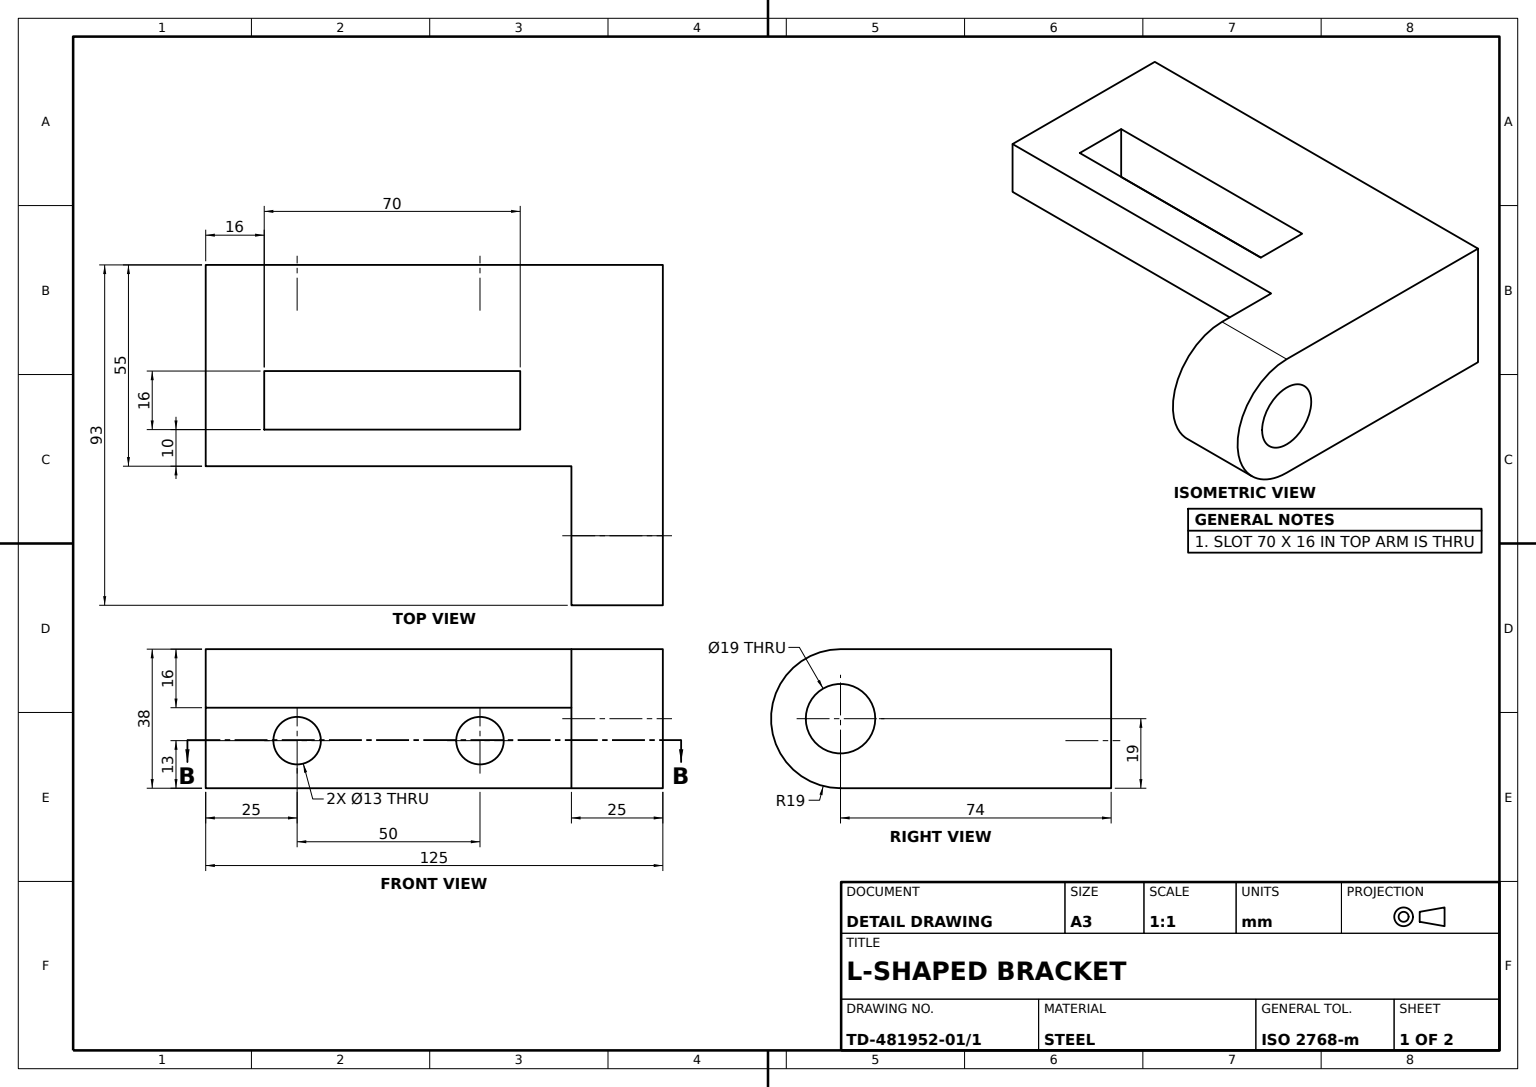
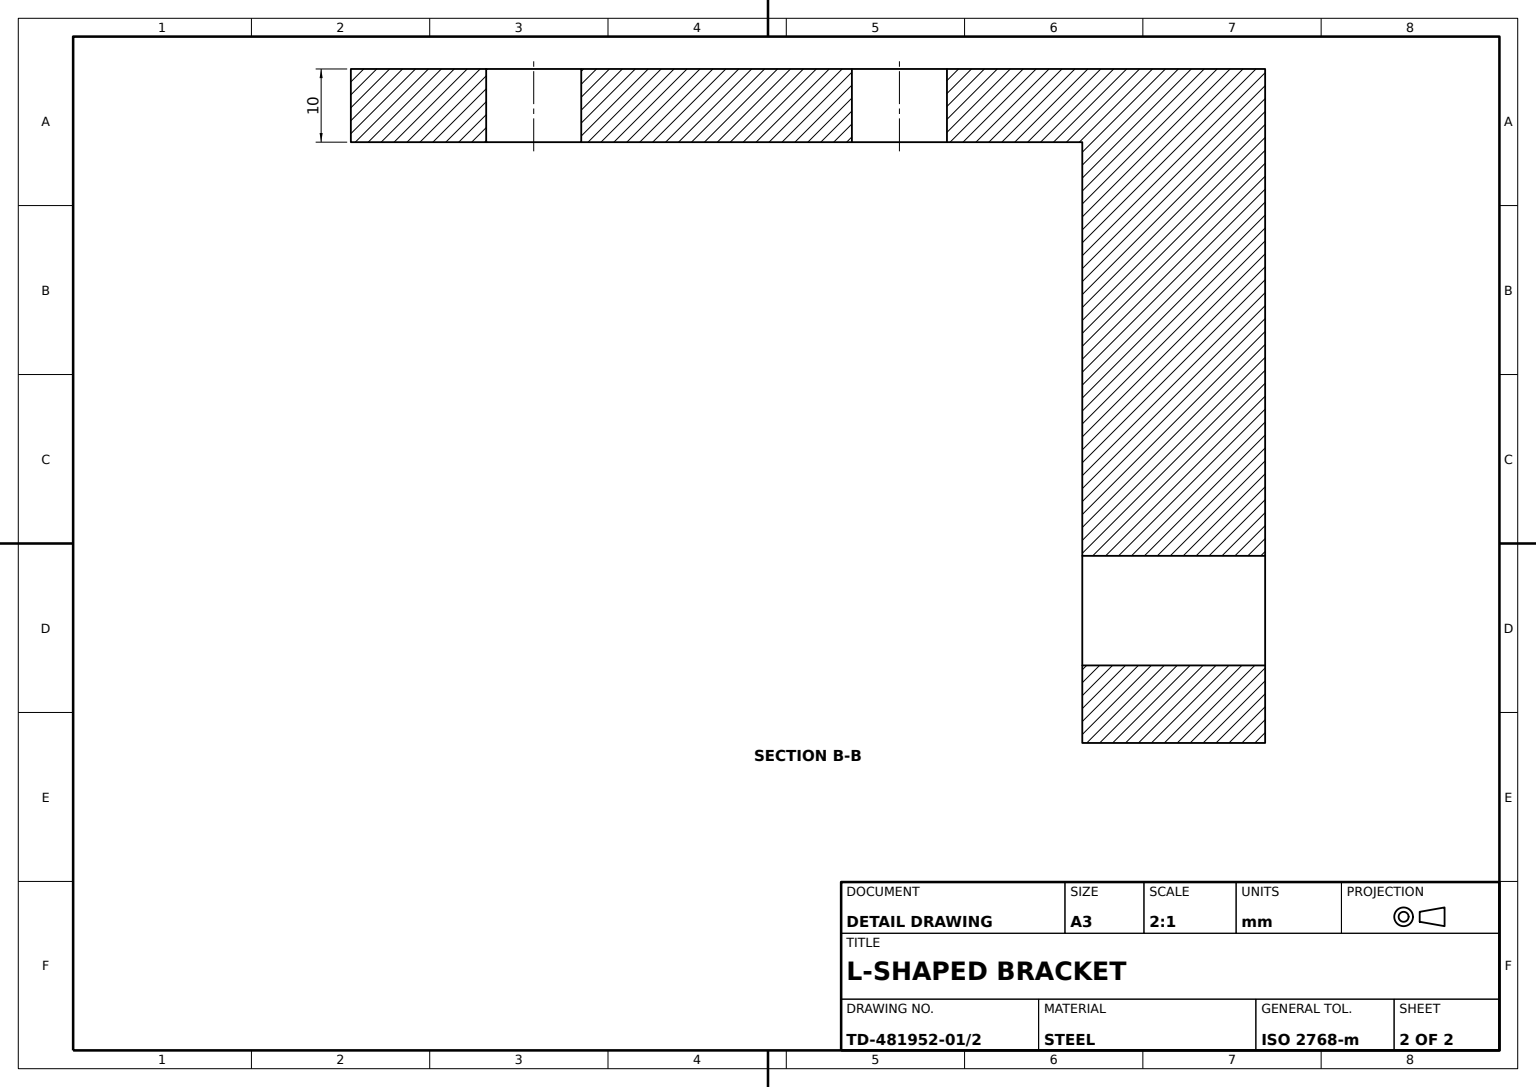
from build123d import *

# Parameters (mm, degrees)
BASE_PLATE_SKETCH_W   = 125
BASE_PLATE_SKETCH_H   = 38
BASE_PLATE_DEPTH      = 10
HINGE_LUG_DEPTH       = 25
LUG_BORE_19_SKETCH_R  = 9.5
LUG_BORE_19_DEPTH     = 25
ARM_SKETCH_W          = 100
ARM_SKETCH_H          = 45
ARM_DEPTH             = 16
SLOT_70X16_SKETCH_W   = 70
SLOT_70X16_SKETCH_H   = 16
SLOT_70X16_DEPTH      = 16
CORNER_NOTCH_SKETCH_R = 6.5
CORNER_NOTCH_DEPTH    = 10


with BuildPart() as part:
    # Base Plate Sketch → Base Plate (new body)
    with BuildSketch(Plane.XY):
        with Locations((62.5, 19)):
            Rectangle(BASE_PLATE_SKETCH_W, BASE_PLATE_SKETCH_H)
    extrude(amount=BASE_PLATE_DEPTH)

    # Hinge Lug Sketch → Hinge Lug (add)
    with BuildSketch(Plane(origin=(125, 0, 0), x_dir=(0, 0, -1), z_dir=(1, 0, 0))):
        with BuildLine():
            Line((-10, 38), (-74, 38))
            ThreePointArc((-74, 38), (-93, 19), (-74, 0))
            Line((-74, 0), (-10, 0))
            Line((-10, 0), (-10, 38))
        make_face()
    extrude(amount=-HINGE_LUG_DEPTH)

    # Lug Bore Ø19 Sketch → Lug Bore Ø19 (cut)
    with BuildSketch(Plane(origin=(125, 0, 0), x_dir=(0, 0, -1), z_dir=(1, 0, 0))):
        with Locations((-74, 19)):
            Circle(LUG_BORE_19_SKETCH_R)
    extrude(amount=-LUG_BORE_19_DEPTH, mode=Mode.SUBTRACT)

    # Arm Sketch → Arm (add)
    with BuildSketch(Plane(origin=(0, 38, 0), x_dir=(1, 0, 0), z_dir=(0, 1, 0))):
        with Locations((50, -32.5)):
            Rectangle(ARM_SKETCH_W, ARM_SKETCH_H)
    extrude(amount=-ARM_DEPTH)

    # Slot 70x16 Sketch → Slot 70x16 (cut)
    with BuildSketch(Plane(origin=(0, 38, 0), x_dir=(1, 0, 0), z_dir=(0, 1, 0))):
        with Locations((51, -37)):
            Rectangle(SLOT_70X16_SKETCH_W, SLOT_70X16_SKETCH_H)
    extrude(amount=-SLOT_70X16_DEPTH, mode=Mode.SUBTRACT)

    # Corner Notch Sketch → Corner Notch (cut)
    with BuildSketch(Plane.XY.offset(10)):
        with Locations((25, 13)):
            Circle(CORNER_NOTCH_SKETCH_R)
        with Locations((75, 13)):
            Circle(CORNER_NOTCH_SKETCH_R)
    extrude(amount=-CORNER_NOTCH_DEPTH, mode=Mode.SUBTRACT)


solid = part.part
